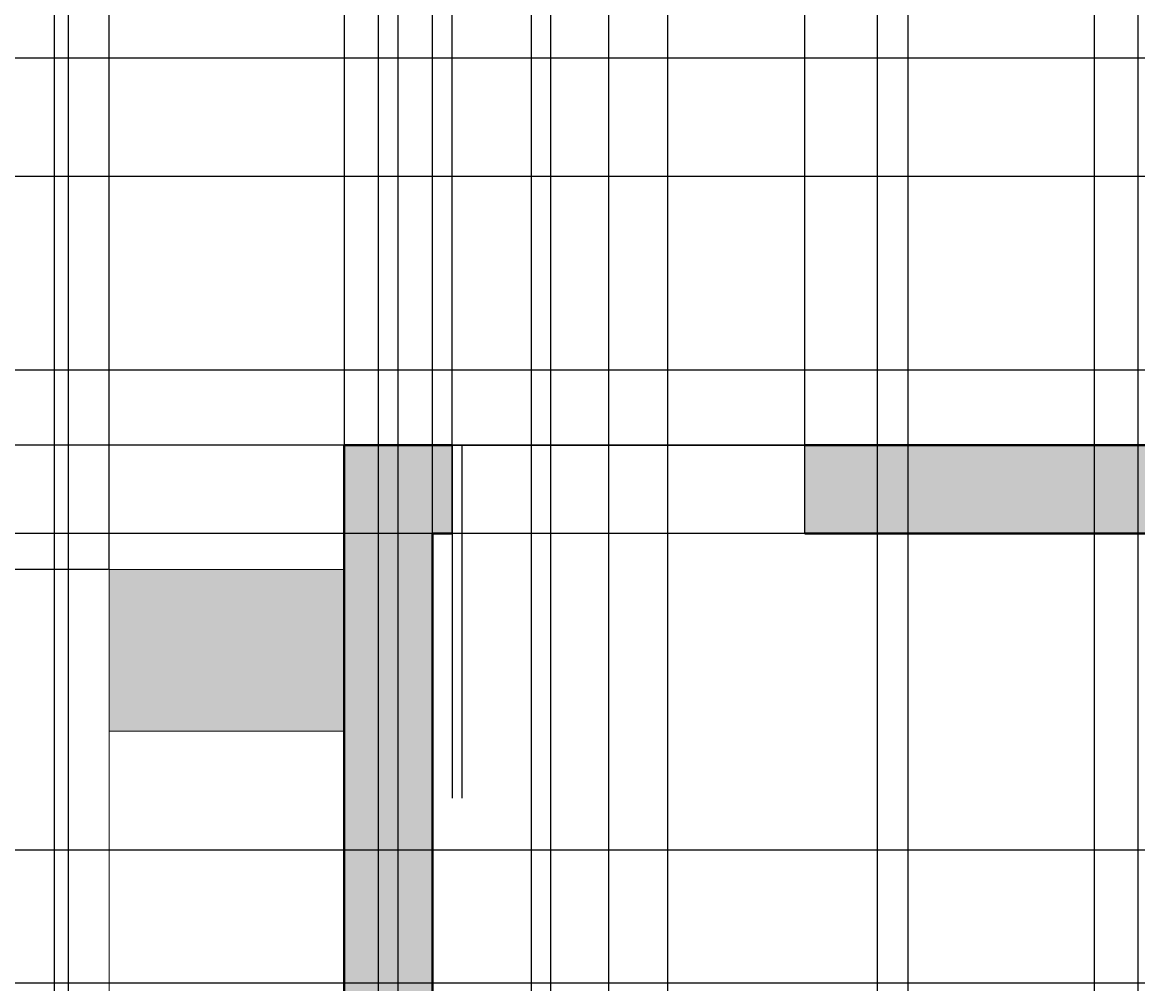
# Model space of a CAD drawing. Units: inches. Extents: x 818 to 1898, y 976 to 2364.
# Tile 27 of 96: x 1398 to 1512, y 1545 to 1643. Entities that reach past the tile are written whole.
import ezdxf

# ---------------------------------------------------------------- set-up
doc = ezdxf.new("R2010")
doc.units = ezdxf.units.IN
doc.header["$LTSCALE"] = 5
doc.header["$MEASUREMENT"] = 0
for name, color, linetype, lineweight in [('A-ANNO-DIMS', 2, 'Continuous', 18), ('A-DOOR', 3, 'Continuous', 25), ('A-FLOR-CASE', 8, 'Continuous', 18), ('A-FURN-PATT', 8, 'Continuous', 9), ('A-WALL', 7, 'Continuous', 40)]:
    doc.layers.add(name, color=color, linetype=linetype, lineweight=lineweight)
doc.layers.add('A-WALL-PATT', color=251, linetype='Continuous', lineweight=13, true_color=0x636466)
doc.styles.get("Standard").update_dxf_attribs({"font": 'arial.ttf'})
doc.dimstyles.get("Standard").update_dxf_attribs({"dimtxt": 0.18, "dimasz": 0.18, "dimexe": 0.18, "dimexo": 0.0625, "dimgap": 0.09, "dimtad": 0, "dimtih": 1, "dimtoh": 1, "dimdec": 4, "dimzin": 0, "dimdsep": 46, "dimtxsty": 'Standard', "dimcen": 0.09, "dimadec": 0, "dimazin": 0, "dimtfac": 1, "dimtdec": 4, "dimtofl": 0, "dimtmove": 0, "dimatfit": 3, "dimfxl": 1, "dimtolj": 1, "dimtzin": 0, "dimarcsym": 0})

# ---------------------------------------------------------------- blocks, each defined once
blk = doc.blocks.new('*D61')
at = {"layer": 'A-ANNO-DIMS', "color": 0, "lineweight": -2, "ltscale": 5, "transparency": 16777216}
for p, q in [((1071.73, 1203.03), (1071.73, 2363.87)), ((1071.91, 2363.69), (1250.94, 2363.69)), ((1430.55, 2363.69), (1251.51, 2363.69)), ((1430.73, 1203.03), (1430.73, 2363.87))]:
    blk.add_line(p, q, dxfattribs=at)
at = {"layer": 'A-ANNO-DIMS', "color": 0, "ltscale": 5, "transparency": 16777216}
for points in [[(1071.91, 2363.72), (1071.91, 2363.66), (1071.73, 2363.69)], [(1430.55, 2363.72), (1430.55, 2363.66), (1430.73, 2363.69)]]:
    blk.add_solid(points, dxfattribs=at)
at = {"layer": 'Defpoints', "color": 0, "ltscale": 5, "transparency": 16777216}
for p in [(1430.73, 2363.69), (1071.73, 1202.96), (1430.73, 1202.96)]:
    blk.add_point(p, dxfattribs=at)
at = {"layer": 'A-ANNO-DIMS', "color": 0, "ltscale": 5, "transparency": 16777216, "insert": (1251.23, 2363.69), "char_height": 0.18, "attachment_point": 5}
blk.add_mtext('\\A1;359', dxfattribs=at)
blk = doc.blocks.new('*D64')
at = {"layer": 'A-ANNO-DIMS', "color": 0, "lineweight": -2, "ltscale": 5, "transparency": 16777216}
for p, q in [((1197.73, 1501.14), (1197.73, 2363.87)), ((1197.91, 2363.69), (1313.93, 2363.69)), ((1430.55, 2363.69), (1314.52, 2363.69)), ((1430.73, 1501.14), (1430.73, 2363.87))]:
    blk.add_line(p, q, dxfattribs=at)
at = {"layer": 'A-ANNO-DIMS', "color": 0, "ltscale": 5, "transparency": 16777216}
for points in [[(1197.91, 2363.72), (1197.91, 2363.66), (1197.73, 2363.69)], [(1430.55, 2363.72), (1430.55, 2363.66), (1430.73, 2363.69)]]:
    blk.add_solid(points, dxfattribs=at)
at = {"layer": 'Defpoints', "color": 0, "ltscale": 5, "transparency": 16777216}
for p in [(1430.73, 2363.69), (1197.73, 1501.08), (1430.73, 1501.08)]:
    blk.add_point(p, dxfattribs=at)
at = {"layer": 'A-ANNO-DIMS', "color": 0, "ltscale": 5, "transparency": 16777216, "insert": (1314.23, 2363.69), "char_height": 0.18, "attachment_point": 5}
blk.add_mtext('\\A1;233', dxfattribs=at)
blk = doc.blocks.new('*D99')
at = {"layer": 'A-ANNO-DIMS', "color": 0, "lineweight": -2, "ltscale": 5, "transparency": 16777216}
for p, q in [((1391.88, 1071.12), (1391.88, 2363.87)), ((1392.06, 2363.69), (1420.45, 2363.69)), ((1449.64, 2363.69), (1421.24, 2363.69)), ((1449.82, 1071.12), (1449.82, 2363.87))]:
    blk.add_line(p, q, dxfattribs=at)
at = {"layer": 'A-ANNO-DIMS', "color": 0, "ltscale": 5, "transparency": 16777216}
for points in [[(1392.06, 2363.72), (1392.06, 2363.66), (1391.88, 2363.69)], [(1449.64, 2363.72), (1449.64, 2363.66), (1449.82, 2363.69)]]:
    blk.add_solid(points, dxfattribs=at)
at = {"layer": 'Defpoints', "color": 0, "ltscale": 5, "transparency": 16777216}
for p in [(1449.82, 2363.69), (1391.88, 1071.06), (1449.82, 1071.06)]:
    blk.add_point(p, dxfattribs=at)
at = {"layer": 'A-ANNO-DIMS', "color": 0, "ltscale": 5, "transparency": 16777216, "insert": (1420.85, 2363.69), "char_height": 0.18, "attachment_point": 5}
blk.add_mtext('\\A1;57.94', dxfattribs=at)
blk = doc.blocks.new('*D100')
at = {"layer": 'A-ANNO-DIMS', "color": 0, "lineweight": -2, "ltscale": 5, "transparency": 16777216}
for p, q in [((1449.82, 1071.12), (1449.82, 2363.87)), ((1450, 2363.69), (1478.17, 2363.69)), ((1507.12, 2363.69), (1478.95, 2363.69)), ((1507.3, 1071.12), (1507.3, 2363.87))]:
    blk.add_line(p, q, dxfattribs=at)
at = {"layer": 'A-ANNO-DIMS', "color": 0, "ltscale": 5, "transparency": 16777216}
for points in [[(1450, 2363.72), (1450, 2363.66), (1449.82, 2363.69)], [(1507.12, 2363.72), (1507.12, 2363.66), (1507.3, 2363.69)]]:
    blk.add_solid(points, dxfattribs=at)
at = {"layer": 'Defpoints', "color": 0, "ltscale": 5, "transparency": 16777216}
for p in [(1507.3, 2363.69), (1449.82, 1071.06), (1507.3, 1071.06)]:
    blk.add_point(p, dxfattribs=at)
at = {"layer": 'A-ANNO-DIMS', "color": 0, "ltscale": 5, "transparency": 16777216, "insert": (1478.56, 2363.69), "char_height": 0.18, "attachment_point": 5}
blk.add_mtext('\\A1;57.48', dxfattribs=at)
blk = doc.blocks.new('*D101')
at = {"layer": 'A-ANNO-DIMS', "color": 0, "lineweight": -2, "ltscale": 5, "transparency": 16777216}
for p, q in [((1507.3, 1071.12), (1507.3, 2363.87)), ((1507.48, 2363.69), (1536, 2363.69)), ((1565.3, 2363.69), (1536.78, 2363.69)), ((1565.48, 1071.12), (1565.48, 2363.87))]:
    blk.add_line(p, q, dxfattribs=at)
at = {"layer": 'A-ANNO-DIMS', "color": 0, "ltscale": 5, "transparency": 16777216}
for points in [[(1507.48, 2363.72), (1507.48, 2363.66), (1507.3, 2363.69)], [(1565.3, 2363.72), (1565.3, 2363.66), (1565.48, 2363.69)]]:
    blk.add_solid(points, dxfattribs=at)
at = {"layer": 'Defpoints', "color": 0, "ltscale": 5, "transparency": 16777216}
for p in [(1565.48, 2363.69), (1507.3, 1071.06), (1565.48, 1071.06)]:
    blk.add_point(p, dxfattribs=at)
at = {"layer": 'A-ANNO-DIMS', "color": 0, "ltscale": 5, "transparency": 16777216, "insert": (1536.39, 2363.69), "char_height": 0.18, "attachment_point": 5}
blk.add_mtext('\\A1;58.19', dxfattribs=at)
blk = doc.blocks.new('*D117')
at = {"layer": 'A-ANNO-DIMS', "color": 0, "lineweight": -2, "ltscale": 5, "transparency": 16777216}
for p, q in [((1766.29, 1545.18), (818.03, 1545.18)), ((818.21, 1545), (818.21, 1501.18)), ((818.21, 1456.99), (818.21, 1500.81)), ((1766.29, 1456.81), (818.03, 1456.81))]:
    blk.add_line(p, q, dxfattribs=at)
at = {"layer": 'A-ANNO-DIMS', "color": 0, "ltscale": 5, "transparency": 16777216}
for points in [[(818.18, 1545), (818.24, 1545), (818.21, 1545.18)], [(818.18, 1456.99), (818.24, 1456.99), (818.21, 1456.81)]]:
    blk.add_solid(points, dxfattribs=at)
at = {"layer": 'Defpoints', "color": 0, "ltscale": 5, "transparency": 16777216}
for p in [(818.21, 1545.18), (1766.35, 1545.18), (1766.35, 1456.81)]:
    blk.add_point(p, dxfattribs=at)
at = {"layer": 'A-ANNO-DIMS', "color": 0, "ltscale": 5, "transparency": 16777216, "insert": (818.21, 1501), "char_height": 0.18, "attachment_point": 5}
blk.add_mtext('\\A1;88.37', dxfattribs=at)
blk = doc.blocks.new('*D118')
at = {"layer": 'A-ANNO-DIMS', "color": 0, "lineweight": -2, "ltscale": 5, "transparency": 16777216}
for p, q in [((1766.29, 1627.51), (818.03, 1627.51)), ((818.21, 1627.33), (818.21, 1586.53)), ((818.21, 1545.36), (818.21, 1586.16)), ((1766.29, 1545.18), (818.03, 1545.18))]:
    blk.add_line(p, q, dxfattribs=at)
at = {"layer": 'A-ANNO-DIMS', "color": 0, "ltscale": 5, "transparency": 16777216}
for points in [[(818.18, 1627.33), (818.24, 1627.33), (818.21, 1627.51)], [(818.18, 1545.36), (818.24, 1545.36), (818.21, 1545.18)]]:
    blk.add_solid(points, dxfattribs=at)
at = {"layer": 'Defpoints', "color": 0, "ltscale": 5, "transparency": 16777216}
for p in [(818.21, 1627.51), (1766.35, 1627.51), (1766.35, 1545.18)]:
    blk.add_point(p, dxfattribs=at)
at = {"layer": 'A-ANNO-DIMS', "color": 0, "ltscale": 5, "transparency": 16777216, "insert": (818.21, 1586.34), "char_height": 0.18, "attachment_point": 5}
blk.add_mtext('\\A1;82.32', dxfattribs=at)
blk = doc.blocks.new('*D119')
at = {"layer": 'A-ANNO-DIMS', "color": 0, "lineweight": -2, "ltscale": 5, "transparency": 16777216}
for p, q in [((1766.29, 1716.99), (818.03, 1716.99)), ((818.21, 1716.81), (818.21, 1672.43)), ((818.21, 1627.69), (818.21, 1672.06)), ((1766.29, 1627.51), (818.03, 1627.51))]:
    blk.add_line(p, q, dxfattribs=at)
at = {"layer": 'A-ANNO-DIMS', "color": 0, "ltscale": 5, "transparency": 16777216}
for points in [[(818.18, 1716.81), (818.24, 1716.81), (818.21, 1716.99)], [(818.18, 1627.69), (818.24, 1627.69), (818.21, 1627.51)]]:
    blk.add_solid(points, dxfattribs=at)
at = {"layer": 'Defpoints', "color": 0, "ltscale": 5, "transparency": 16777216}
for p in [(818.21, 1716.99), (1766.35, 1716.99), (1766.35, 1627.51)]:
    blk.add_point(p, dxfattribs=at)
at = {"layer": 'A-ANNO-DIMS', "color": 0, "ltscale": 5, "transparency": 16777216, "insert": (818.21, 1672.25), "char_height": 0.18, "attachment_point": 5}
blk.add_mtext('\\A1;89.48', dxfattribs=at)
blk = doc.blocks.new('*D159')
at = {"layer": 'A-ANNO-DIMS', "color": 0, "lineweight": -2, "ltscale": 5, "transparency": 16777216}
for p, q in [((1206.73, 1687.02), (1206.73, 975.66)), ((1463.73, 1687.02), (1463.73, 975.66)), ((1206.91, 975.84), (1334.93, 975.84)), ((1463.55, 975.84), (1335.52, 975.84))]:
    blk.add_line(p, q, dxfattribs=at)
at = {"layer": 'A-ANNO-DIMS', "color": 0, "ltscale": 5, "transparency": 16777216}
for points in [[(1206.91, 975.87), (1206.91, 975.81), (1206.73, 975.84)], [(1463.55, 975.87), (1463.55, 975.81), (1463.73, 975.84)]]:
    blk.add_solid(points, dxfattribs=at)
at = {"layer": 'Defpoints', "color": 0, "ltscale": 5, "transparency": 16777216}
for p in [(1206.73, 1687.08), (1463.73, 1687.08), (1463.73, 975.84)]:
    blk.add_point(p, dxfattribs=at)
at = {"layer": 'A-ANNO-DIMS', "color": 0, "ltscale": 5, "transparency": 16777216, "insert": (1335.23, 975.84), "char_height": 0.18, "attachment_point": 5}
blk.add_mtext('\\A1;257', dxfattribs=at)
blk = doc.blocks.new('*D160')
at = {"layer": 'A-ANNO-DIMS', "color": 0, "lineweight": -2, "ltscale": 5, "transparency": 16777216}
for p, q in [((1463.73, 1687.02), (1463.73, 975.66)), ((1511.73, 1687.02), (1511.73, 975.66)), ((1463.91, 975.84), (1487.5, 975.84)), ((1511.55, 975.84), (1487.95, 975.84))]:
    blk.add_line(p, q, dxfattribs=at)
at = {"layer": 'A-ANNO-DIMS', "color": 0, "ltscale": 5, "transparency": 16777216}
for points in [[(1463.91, 975.87), (1463.91, 975.81), (1463.73, 975.84)], [(1511.55, 975.87), (1511.55, 975.81), (1511.73, 975.84)]]:
    blk.add_solid(points, dxfattribs=at)
at = {"layer": 'Defpoints', "color": 0, "ltscale": 5, "transparency": 16777216}
for p in [(1463.73, 1687.08), (1511.73, 1687.08), (1511.73, 975.84)]:
    blk.add_point(p, dxfattribs=at)
at = {"layer": 'A-ANNO-DIMS', "color": 0, "ltscale": 5, "transparency": 16777216, "insert": (1487.73, 975.84), "char_height": 0.18, "attachment_point": 5}
blk.add_mtext('\\A1;48', dxfattribs=at)
blk = doc.blocks.new('*D166')
at = {"layer": 'A-ANNO-DIMS', "color": 0, "lineweight": -2, "ltscale": 5, "transparency": 16777216}
for p, q in [((1401.15, 1510.14), (1401.15, 2363.87)), ((1401.33, 2363.69), (1415.54, 2363.69)), ((1430.55, 2363.69), (1416.33, 2363.69)), ((1430.73, 1510.14), (1430.73, 2363.87))]:
    blk.add_line(p, q, dxfattribs=at)
at = {"layer": 'A-ANNO-DIMS', "color": 0, "ltscale": 5, "transparency": 16777216}
for points in [[(1401.33, 2363.72), (1401.33, 2363.66), (1401.15, 2363.69)], [(1430.55, 2363.72), (1430.55, 2363.66), (1430.73, 2363.69)]]:
    blk.add_solid(points, dxfattribs=at)
at = {"layer": 'Defpoints', "color": 0, "ltscale": 5, "transparency": 16777216}
for p in [(1430.73, 2363.69), (1401.15, 1510.08), (1430.73, 1510.08)]:
    blk.add_point(p, dxfattribs=at)
at = {"layer": 'A-ANNO-DIMS', "color": 0, "ltscale": 5, "transparency": 16777216, "insert": (1415.94, 2363.69), "char_height": 0.18, "attachment_point": 5}
blk.add_mtext('\\A1;29.58', dxfattribs=at)
blk = doc.blocks.new('*D169')
at = {"layer": 'A-ANNO-DIMS', "color": 0, "lineweight": -2, "ltscale": 5, "transparency": 16777216}
for p, q in [((1441.73, 1600.14), (1441.73, 2363.87)), ((1441.91, 2363.69), (1459.51, 2363.69)), ((1477.55, 2363.69), (1459.94, 2363.69)), ((1477.73, 1600.14), (1477.73, 2363.87))]:
    blk.add_line(p, q, dxfattribs=at)
at = {"layer": 'A-ANNO-DIMS', "color": 0, "ltscale": 5, "transparency": 16777216}
for points in [[(1441.91, 2363.72), (1441.91, 2363.66), (1441.73, 2363.69)], [(1477.55, 2363.72), (1477.55, 2363.66), (1477.73, 2363.69)]]:
    blk.add_solid(points, dxfattribs=at)
at = {"layer": 'Defpoints', "color": 0, "ltscale": 5, "transparency": 16777216}
for p in [(1477.73, 2363.69), (1441.73, 1600.08), (1477.73, 1600.08)]:
    blk.add_point(p, dxfattribs=at)
at = {"layer": 'A-ANNO-DIMS', "color": 0, "ltscale": 5, "transparency": 16777216, "insert": (1459.73, 2363.69), "char_height": 0.18, "attachment_point": 5}
blk.add_mtext('\\A1;36', dxfattribs=at)
blk = doc.blocks.new('*D170')
at = {"layer": 'A-ANNO-DIMS', "color": 0, "lineweight": -2, "ltscale": 5, "transparency": 16777216}
for p, q in [((1430.79, 1600.08), (1897.92, 1600.08)), ((1897.74, 1599.9), (1897.74, 1550.76)), ((1897.74, 1501.26), (1897.74, 1550.4)), ((1430.79, 1501.08), (1897.92, 1501.08))]:
    blk.add_line(p, q, dxfattribs=at)
at = {"layer": 'A-ANNO-DIMS', "color": 0, "ltscale": 5, "transparency": 16777216}
for points in [[(1897.71, 1599.9), (1897.77, 1599.9), (1897.74, 1600.08)], [(1897.71, 1501.26), (1897.77, 1501.26), (1897.74, 1501.08)]]:
    blk.add_solid(points, dxfattribs=at)
at = {"layer": 'Defpoints', "color": 0, "ltscale": 5, "transparency": 16777216}
for p in [(1430.73, 1600.08), (1897.74, 1600.08), (1430.73, 1501.08)]:
    blk.add_point(p, dxfattribs=at)
at = {"layer": 'A-ANNO-DIMS', "color": 0, "ltscale": 5, "transparency": 16777216, "insert": (1897.74, 1550.58), "char_height": 0.18, "attachment_point": 5}
blk.add_mtext('\\A1;99', dxfattribs=at)
blk = doc.blocks.new('*D181')
at = {"layer": 'A-ANNO-DIMS', "color": 0, "lineweight": -2, "ltscale": 5, "transparency": 16777216}
for p, q in [((1599.66, 1639.58), (818.03, 1639.58)), ((818.21, 1639.4), (818.21, 1620.01)), ((818.21, 1600.26), (818.21, 1619.65)), ((1619.66, 1600.08), (818.03, 1600.08))]:
    blk.add_line(p, q, dxfattribs=at)
at = {"layer": 'A-ANNO-DIMS', "color": 0, "ltscale": 5, "transparency": 16777216}
for points in [[(818.18, 1639.4), (818.24, 1639.4), (818.21, 1639.58)], [(818.18, 1600.26), (818.24, 1600.26), (818.21, 1600.08)]]:
    blk.add_solid(points, dxfattribs=at)
at = {"layer": 'Defpoints', "color": 0, "ltscale": 5, "transparency": 16777216}
for p in [(1599.73, 1639.58), (818.21, 1600.08), (1619.73, 1600.08)]:
    blk.add_point(p, dxfattribs=at)
at = {"layer": 'A-ANNO-DIMS', "color": 0, "ltscale": 5, "transparency": 16777216, "insert": (818.21, 1619.83), "char_height": 0.18, "attachment_point": 5}
blk.add_mtext('\\A1;39.5', dxfattribs=at)
blk = doc.blocks.new('*D182')
at = {"layer": 'A-ANNO-DIMS', "color": 0, "lineweight": -2, "ltscale": 5, "transparency": 16777216}
for p, q in [((1463.73, 1687.02), (1463.73, 975.66)), ((1559.73, 1687.02), (1559.73, 975.66)), ((1463.91, 975.84), (1511.51, 975.84)), ((1559.55, 975.84), (1511.94, 975.84))]:
    blk.add_line(p, q, dxfattribs=at)
at = {"layer": 'A-ANNO-DIMS', "color": 0, "ltscale": 5, "transparency": 16777216}
for points in [[(1463.91, 975.87), (1463.91, 975.81), (1463.73, 975.84)], [(1559.55, 975.87), (1559.55, 975.81), (1559.73, 975.84)]]:
    blk.add_solid(points, dxfattribs=at)
at = {"layer": 'Defpoints', "color": 0, "ltscale": 5, "transparency": 16777216}
for p in [(1463.73, 1687.08), (1559.73, 1687.08), (1559.73, 975.84)]:
    blk.add_point(p, dxfattribs=at)
at = {"layer": 'A-ANNO-DIMS', "color": 0, "ltscale": 5, "transparency": 16777216, "insert": (1511.73, 975.84), "char_height": 0.18, "attachment_point": 5}
blk.add_mtext('\\A1;96', dxfattribs=at)
blk = doc.blocks.new('*D191')
at = {"layer": 'A-ANNO-DIMS', "color": 0, "lineweight": -2, "ltscale": 5, "transparency": 16777216}
for p, q in [((1434.23, 1409.11), (1434.23, 2363.87)), ((1434.41, 2363.69), (1435.08, 2363.69)), ((1436.05, 2363.69), (1435.37, 2363.69)), ((1436.23, 1409.11), (1436.23, 2363.87))]:
    blk.add_line(p, q, dxfattribs=at)
at = {"layer": 'A-ANNO-DIMS', "color": 0, "ltscale": 5, "transparency": 16777216}
for points in [[(1434.41, 2363.72), (1434.41, 2363.66), (1434.23, 2363.69)], [(1436.05, 2363.72), (1436.05, 2363.66), (1436.23, 2363.69)]]:
    blk.add_solid(points, dxfattribs=at)
at = {"layer": 'Defpoints', "color": 0, "ltscale": 5, "transparency": 16777216}
for p in [(1436.23, 2363.69), (1434.23, 1409.05), (1436.23, 1409.05)]:
    blk.add_point(p, dxfattribs=at)
at = {"layer": 'A-ANNO-DIMS', "color": 0, "ltscale": 5, "transparency": 16777216, "insert": (1435.23, 2363.69), "char_height": 0.18, "attachment_point": 5}
blk.add_mtext('\\A1;2', dxfattribs=at)
blk = doc.blocks.new('*D194')
at = {"layer": 'A-ANNO-DIMS', "color": 0, "lineweight": -2, "ltscale": 5, "transparency": 16777216}
for p, q in [((1616.66, 1591.08), (818.03, 1591.08)), ((818.21, 1590.9), (818.21, 1575.1)), ((818.21, 1558.93), (818.21, 1574.73)), ((1616.66, 1558.75), (818.03, 1558.75))]:
    blk.add_line(p, q, dxfattribs=at)
at = {"layer": 'A-ANNO-DIMS', "color": 0, "ltscale": 5, "transparency": 16777216}
for points in [[(818.18, 1590.9), (818.24, 1590.9), (818.21, 1591.08)], [(818.18, 1558.93), (818.24, 1558.93), (818.21, 1558.75)]]:
    blk.add_solid(points, dxfattribs=at)
at = {"layer": 'Defpoints', "color": 0, "ltscale": 5, "transparency": 16777216}
for p in [(818.21, 1591.08), (1616.73, 1591.08), (1616.73, 1558.75)]:
    blk.add_point(p, dxfattribs=at)
at = {"layer": 'A-ANNO-DIMS', "color": 0, "ltscale": 5, "transparency": 16777216, "insert": (818.21, 1574.92), "char_height": 0.18, "attachment_point": 5}
blk.add_mtext('\\A1;32.326', dxfattribs=at)
blk = doc.blocks.new('*D196')
at = {"layer": 'A-ANNO-DIMS', "color": 0, "lineweight": -2, "ltscale": 5, "transparency": 16777216}
for p, q in [((1439.73, 1526.73), (1439.73, 2363.87)), ((1439.91, 2363.69), (1448.51, 2363.69)), ((1457.55, 2363.69), (1448.94, 2363.69)), ((1457.73, 1526.73), (1457.73, 2363.87))]:
    blk.add_line(p, q, dxfattribs=at)
at = {"layer": 'A-ANNO-DIMS', "color": 0, "ltscale": 5, "transparency": 16777216}
for points in [[(1439.91, 2363.72), (1439.91, 2363.66), (1439.73, 2363.69)], [(1457.55, 2363.72), (1457.55, 2363.66), (1457.73, 2363.69)]]:
    blk.add_solid(points, dxfattribs=at)
at = {"layer": 'Defpoints', "color": 0, "ltscale": 5, "transparency": 16777216}
for p in [(1457.73, 2363.69), (1439.73, 1526.67), (1457.73, 1526.67)]:
    blk.add_point(p, dxfattribs=at)
at = {"layer": 'A-ANNO-DIMS', "color": 0, "ltscale": 5, "transparency": 16777216, "insert": (1448.73, 2363.69), "char_height": 0.18, "attachment_point": 5}
blk.add_mtext('\\A1;18', dxfattribs=at)
blk = doc.blocks.new('*D214')
at = {"layer": 'A-ANNO-DIMS', "color": 0, "lineweight": -2, "ltscale": 5, "transparency": 16777216}
for p, q in [((1511.73, 1687.02), (1511.73, 975.66)), ((1714.73, 1687.02), (1714.73, 975.66)), ((1511.91, 975.84), (1612.93, 975.84)), ((1714.55, 975.84), (1613.52, 975.84))]:
    blk.add_line(p, q, dxfattribs=at)
at = {"layer": 'A-ANNO-DIMS', "color": 0, "ltscale": 5, "transparency": 16777216}
for points in [[(1511.91, 975.87), (1511.91, 975.81), (1511.73, 975.84)], [(1714.55, 975.87), (1714.55, 975.81), (1714.73, 975.84)]]:
    blk.add_solid(points, dxfattribs=at)
at = {"layer": 'Defpoints', "color": 0, "ltscale": 5, "transparency": 16777216}
for p in [(1511.73, 1687.08), (1714.73, 1687.08), (1714.73, 975.84)]:
    blk.add_point(p, dxfattribs=at)
at = {"layer": 'A-ANNO-DIMS', "color": 0, "ltscale": 5, "transparency": 16777216, "insert": (1613.23, 975.84), "char_height": 0.18, "attachment_point": 5}
blk.add_mtext('\\A1;203', dxfattribs=at)
blk = doc.blocks.new('*D231')
at = {"layer": 'A-ANNO-DIMS', "color": 0, "lineweight": -2, "ltscale": 5, "transparency": 16777216}
for p, q in [((1303.93, 1952.98), (1303.93, 975.66)), ((1402.52, 1952.98), (1402.52, 975.66)), ((1304.11, 975.84), (1352.83, 975.84)), ((1402.34, 975.84), (1353.62, 975.84))]:
    blk.add_line(p, q, dxfattribs=at)
at = {"layer": 'A-ANNO-DIMS', "color": 0, "ltscale": 5, "transparency": 16777216}
for points in [[(1304.11, 975.87), (1304.11, 975.81), (1303.93, 975.84)], [(1402.34, 975.87), (1402.34, 975.81), (1402.52, 975.84)]]:
    blk.add_solid(points, dxfattribs=at)
at = {"layer": 'Defpoints', "color": 0, "ltscale": 5, "transparency": 16777216}
for p in [(1303.93, 1953.04), (1402.52, 1953.04), (1402.52, 975.84)]:
    blk.add_point(p, dxfattribs=at)
at = {"layer": 'A-ANNO-DIMS', "color": 0, "ltscale": 5, "transparency": 16777216, "insert": (1353.22, 975.84), "char_height": 0.18, "attachment_point": 5}
blk.add_mtext('\\A1;98.59', dxfattribs=at)
blk = doc.blocks.new('*D242')
at = {"layer": 'A-ANNO-DIMS', "color": 0, "lineweight": -2, "ltscale": 5, "transparency": 16777216}
for p, q in [((1488.26, 1948.6), (1488.26, 975.66)), ((1513.23, 1948.6), (1513.23, 975.66)), ((1488.44, 975.84), (1500.35, 975.84)), ((1513.05, 975.84), (1501.14, 975.84))]:
    blk.add_line(p, q, dxfattribs=at)
at = {"layer": 'A-ANNO-DIMS', "color": 0, "ltscale": 5, "transparency": 16777216}
for points in [[(1488.44, 975.87), (1488.44, 975.81), (1488.26, 975.84)], [(1513.05, 975.87), (1513.05, 975.81), (1513.23, 975.84)]]:
    blk.add_solid(points, dxfattribs=at)
at = {"layer": 'Defpoints', "color": 0, "ltscale": 5, "transparency": 16777216}
for p in [(1488.26, 1948.66), (1513.23, 1948.66), (1513.23, 975.84)]:
    blk.add_point(p, dxfattribs=at)
at = {"layer": 'A-ANNO-DIMS', "color": 0, "ltscale": 5, "transparency": 16777216, "insert": (1500.74, 975.84), "char_height": 0.18, "attachment_point": 5}
blk.add_mtext('\\A1;24.97', dxfattribs=at)
blk = doc.blocks.new('*D243')
at = {"layer": 'A-ANNO-DIMS', "color": 0, "lineweight": -2, "ltscale": 5, "transparency": 16777216}
for p, q in [((1451.77, 2020.02), (1451.77, 975.66)), ((1590.73, 2020.02), (1590.73, 975.66)), ((1451.95, 975.84), (1520.79, 975.84)), ((1590.55, 975.84), (1521.7, 975.84))]:
    blk.add_line(p, q, dxfattribs=at)
at = {"layer": 'A-ANNO-DIMS', "color": 0, "ltscale": 5, "transparency": 16777216}
for points in [[(1451.95, 975.87), (1451.95, 975.81), (1451.77, 975.84)], [(1590.55, 975.87), (1590.55, 975.81), (1590.73, 975.84)]]:
    blk.add_solid(points, dxfattribs=at)
at = {"layer": 'Defpoints', "color": 0, "ltscale": 5, "transparency": 16777216}
for p in [(1451.77, 2020.08), (1590.73, 2020.08), (1590.73, 975.84)]:
    blk.add_point(p, dxfattribs=at)
at = {"layer": 'A-ANNO-DIMS', "color": 0, "ltscale": 5, "transparency": 16777216, "insert": (1521.25, 975.84), "char_height": 0.18, "attachment_point": 5}
blk.add_mtext('\\A1;138.96', dxfattribs=at)
blk = doc.blocks.new('*D253')
at = {"layer": 'A-ANNO-DIMS', "color": 0, "lineweight": -2, "ltscale": 5, "transparency": 16777216}
for p, q in [((1485.12, 2053.02), (1485.12, 975.66)), ((1538.52, 2053.02), (1538.52, 975.66)), ((1485.3, 975.84), (1511.42, 975.84)), ((1538.34, 975.84), (1512.21, 975.84))]:
    blk.add_line(p, q, dxfattribs=at)
at = {"layer": 'A-ANNO-DIMS', "color": 0, "ltscale": 5, "transparency": 16777216}
for points in [[(1485.3, 975.87), (1485.3, 975.81), (1485.12, 975.84)], [(1538.34, 975.87), (1538.34, 975.81), (1538.52, 975.84)]]:
    blk.add_solid(points, dxfattribs=at)
at = {"layer": 'Defpoints', "color": 0, "ltscale": 5, "transparency": 16777216}
for p in [(1485.12, 2053.08), (1538.52, 2053.08), (1538.52, 975.84)]:
    blk.add_point(p, dxfattribs=at)
at = {"layer": 'A-ANNO-DIMS', "color": 0, "ltscale": 5, "transparency": 16777216, "insert": (1511.82, 975.84), "char_height": 0.18, "attachment_point": 5}
blk.add_mtext('\\A1;53.39', dxfattribs=at)
blk = doc.blocks.new('*D272')
at = {"layer": 'A-ANNO-DIMS', "color": 0, "lineweight": -2, "ltscale": 5, "transparency": 16777216}
for p, q in [((1406.66, 1587.42), (818.03, 1587.42)), ((818.21, 1587.24), (818.21, 1556.89)), ((818.21, 1526.18), (818.21, 1556.52)), ((1406.66, 1526), (818.03, 1526))]:
    blk.add_line(p, q, dxfattribs=at)
at = {"layer": 'A-ANNO-DIMS', "color": 0, "ltscale": 5, "transparency": 16777216}
for points in [[(818.18, 1587.24), (818.24, 1587.24), (818.21, 1587.42)], [(818.18, 1526.18), (818.24, 1526.18), (818.21, 1526)]]:
    blk.add_solid(points, dxfattribs=at)
at = {"layer": 'Defpoints', "color": 0, "ltscale": 5, "transparency": 16777216}
for p in [(818.21, 1587.42), (1406.73, 1587.42), (1406.73, 1526)]:
    blk.add_point(p, dxfattribs=at)
at = {"layer": 'A-ANNO-DIMS', "color": 0, "ltscale": 5, "transparency": 16777216, "insert": (818.21, 1556.71), "char_height": 0.18, "attachment_point": 5}
blk.add_mtext('\\A1;61.42', dxfattribs=at)
blk = doc.blocks.new('*D273')
at = {"layer": 'A-ANNO-DIMS', "color": 0, "lineweight": -2, "ltscale": 5, "transparency": 16777216}
for p, q in [((1406.73, 1587.48), (1406.73, 2363.87)), ((1406.91, 2363.69), (1418.51, 2363.69)), ((1430.55, 2363.69), (1418.95, 2363.69)), ((1430.73, 1587.48), (1430.73, 2363.87))]:
    blk.add_line(p, q, dxfattribs=at)
at = {"layer": 'A-ANNO-DIMS', "color": 0, "ltscale": 5, "transparency": 16777216}
for points in [[(1406.91, 2363.72), (1406.91, 2363.66), (1406.73, 2363.69)], [(1430.55, 2363.72), (1430.55, 2363.66), (1430.73, 2363.69)]]:
    blk.add_solid(points, dxfattribs=at)
at = {"layer": 'Defpoints', "color": 0, "ltscale": 5, "transparency": 16777216}
for p in [(1430.73, 2363.69), (1406.73, 1587.42), (1430.73, 1587.42)]:
    blk.add_point(p, dxfattribs=at)
at = {"layer": 'A-ANNO-DIMS', "color": 0, "ltscale": 5, "transparency": 16777216, "insert": (1418.73, 2363.69), "char_height": 0.18, "attachment_point": 5}
blk.add_mtext('\\A1;24', dxfattribs=at)
blk = doc.blocks.new('*D291')
at = {"layer": 'A-ANNO-DIMS', "color": 0, "lineweight": -2, "ltscale": 5, "transparency": 16777216}
for p, q in [((1206.79, 1687.08), (1897.92, 1687.08)), ((1897.74, 1686.9), (1897.74, 1647.61)), ((1897.74, 1607.95), (1897.74, 1647.24)), ((1318.96, 1607.77), (1897.92, 1607.77))]:
    blk.add_line(p, q, dxfattribs=at)
at = {"layer": 'A-ANNO-DIMS', "color": 0, "ltscale": 5, "transparency": 16777216}
for points in [[(1897.71, 1686.9), (1897.77, 1686.9), (1897.74, 1687.08)], [(1897.71, 1607.95), (1897.77, 1607.95), (1897.74, 1607.77)]]:
    blk.add_solid(points, dxfattribs=at)
at = {"layer": 'Defpoints', "color": 0, "ltscale": 5, "transparency": 16777216}
for p in [(1206.73, 1687.08), (1897.74, 1687.08), (1318.89, 1607.77)]:
    blk.add_point(p, dxfattribs=at)
at = {"layer": 'A-ANNO-DIMS', "color": 0, "ltscale": 5, "transparency": 16777216, "insert": (1897.74, 1647.42), "char_height": 0.18, "attachment_point": 5}
blk.add_mtext('\\A1;79.3', dxfattribs=at)

msp = doc.modelspace()

# ---------------------------------------------------------------- hatches: boundary and pattern name
at = {"layer": 'A-FURN-PATT', "ltscale": 5}
h = msp.add_hatch(color=256, dxfattribs=at)
h.dxf.hatch_style = 1
h.paths.add_polyline_path([(1336.7936, 1953.0408), (1314.2595, 1953.0408), (1314.2595, 1941.0096), (1336.7936, 1941.0096)])
h.paths.add_polyline_path([(1338.9915, 1941.0096), (1336.7936, 1941.0096), (1336.7936, 1937.7177), (1314.2595, 1937.7177), (1314.2595, 1941.0096), (1310.9077, 1941.0096), (1310.9077, 1935.2252), (1338.9915, 1935.2252)])
h.paths.add_polyline_path([(1336.7936, 1941.0096), (1314.2595, 1941.0096), (1314.2595, 1937.7177), (1336.7936, 1937.7177)], flags=17)
h.paths.add_polyline_path([(1367.9307, 1959.6079), (1345.3966, 1959.6079), (1345.3966, 1941.0096), (1367.9307, 1941.0096)])
h.paths.add_polyline_path([(1398.8475, 1953.0408), (1376.3134, 1953.0408), (1376.3134, 1952.6393), (1390.1242, 1941.0096), (1398.8475, 1941.0096)])
h.paths.add_polyline_path([(1376.3134, 1952.6393), (1376.3134, 1941.0096), (1390.1242, 1941.0096)], flags=17)
h.paths.add_polyline_path([(1370.1286, 1941.0096), (1367.9307, 1941.0096), (1367.9307, 1937.7177), (1345.3966, 1937.7177), (1345.3966, 1941.0096), (1342.0448, 1941.0096), (1342.0448, 1935.2252), (1370.1286, 1935.2252)])
h.paths.add_polyline_path([(1367.9307, 1941.0096), (1345.3966, 1941.0096), (1345.3966, 1937.7177), (1367.9307, 1937.7177)], flags=17)
h.paths.add_polyline_path([(1390.1242, 1941.0096), (1376.3134, 1941.0096), (1376.3134, 1937.7177), (1394.0336, 1937.7177)], flags=17)
h.paths.add_polyline_path([(1394.0336, 1937.7177), (1376.3134, 1937.7177), (1376.3134, 1941.0096), (1372.9616, 1941.0096), (1372.9616, 1935.2252), (1396.9935, 1935.2252)])
h.paths.add_polyline_path([(1398.8475, 1941.0096), (1390.1242, 1941.0096), (1394.0336, 1937.7177), (1398.8475, 1937.7177)])
h.paths.add_polyline_path([(1401.0455, 1941.0096), (1398.8475, 1941.0096), (1398.8475, 1937.7177), (1394.0336, 1937.7177), (1396.9935, 1935.2252), (1401.0455, 1935.2252)])
h.paths.add_polyline_path([(1336.7936, 2020.4229), (1314.2595, 2020.4229), (1314.2595, 2008.3917), (1336.7936, 2008.3917)])
h.paths.add_polyline_path([(1336.7936, 2023.7149), (1314.2595, 2023.7149), (1314.2595, 2020.4229), (1336.7936, 2020.4229)], flags=17)
h.paths.add_polyline_path([(1338.9915, 2026.2074), (1310.9077, 2026.2074), (1310.9077, 2020.4229), (1314.2595, 2020.4229), (1314.2595, 2023.7149), (1336.7936, 2023.7149), (1336.7936, 2020.4229), (1338.9915, 2020.4229)])
h.paths.add_polyline_path([(1367.9307, 2023.7149), (1345.3966, 2023.7149), (1345.3966, 2020.4229), (1367.9307, 2020.4229)], flags=17)
h.paths.add_polyline_path([(1370.1286, 2026.2074), (1342.0448, 2026.2074), (1342.0448, 2020.4229), (1345.3966, 2020.4229), (1345.3966, 2023.7149), (1367.9307, 2023.7149), (1367.9307, 2020.4229), (1370.1286, 2020.4229)])
h.paths.add_polyline_path([(1367.9307, 2020.4229), (1345.3966, 2020.4229), (1345.3966, 2008.3917), (1367.9307, 2008.3917)])
h.paths.add_polyline_path([(1398.8475, 2020.4229), (1388.1824, 2020.4229), (1376.3134, 2010.4284), (1376.3134, 2008.3917), (1398.8475, 2008.3917)])
h.paths.add_polyline_path([(1392.0918, 2023.7149), (1376.3134, 2023.7149), (1376.3134, 2020.4229), (1388.1824, 2020.4229)], flags=17)
h.paths.add_polyline_path([(1388.1824, 2020.4229), (1376.3134, 2020.4229), (1376.3134, 2010.4284)], flags=17)
h.paths.add_polyline_path([(1395.0518, 2026.2074), (1372.9616, 2026.2074), (1372.9616, 2020.4229), (1376.3134, 2020.4229), (1376.3134, 2023.7149), (1392.0918, 2023.7149)])
h.paths.add_polyline_path([(1398.8475, 2023.7149), (1392.0918, 2023.7149), (1388.1824, 2020.4229), (1398.8475, 2020.4229)])
h.paths.add_polyline_path([(1401.0455, 2026.2074), (1395.0518, 2026.2074), (1392.0918, 2023.7149), (1398.8475, 2023.7149), (1398.8475, 2020.4229), (1401.0455, 2020.4229)])
h.paths.add_polyline_path([(1327.0339, 1897.8663), (1311.025, 1897.8663), (1311.025, 1876.0782), (1327.0339, 1876.0782)])
h.paths.add_polyline_path([(1377.7791, 1897.8663), (1359.9579, 1897.8663), (1359.9579, 1876.0782), (1377.7791, 1876.0782)])
h.paths.add_polyline_path([(1430.7251, 1541.0439), (1406.7251, 1541.0439), (1406.7251, 1525.9965), (1430.7251, 1525.9965)])
h.paths.add_polyline_path([(1430.7251, 1587.4164), (1406.7251, 1587.4164), (1406.7251, 1570.9187), (1430.7251, 1570.9187)])
at = {"layer": 'A-WALL-PATT', "ltscale": 5}
h = msp.add_hatch(color=256, dxfattribs=at)
h.dxf.hatch_style = 1
h.paths.add_polyline_path([(1267.7252, 1928.9218), (1258.7252, 1928.9218), (1258.7252, 1913.6401), (1250.3029, 1913.6401), (1250.3029, 1878.3919), (1258.7252, 1878.3919), (1258.7252, 1862.9652), (1267.7252, 1862.9652)])
h.paths.add_polyline_path([(1267.7252, 1814.9652), (1258.7252, 1814.9652), (1258.7252, 1755.3321), (1267.7252, 1755.3321)])
h.paths.add_polyline_path([(1463.7251, 1696.0782), (1267.7252, 1696.0782), (1267.7252, 1707.3321), (1258.7252, 1707.3321), (1258.7252, 1700.0782), (1251.9333, 1700.0782), (1251.9333, 1687.0782), (1463.7251, 1687.0782)])
h.paths.add_polyline_path([(1714.7251, 1717.3178), (1705.7252, 1717.3178), (1705.7252, 1696.0782), (1599.7251, 1696.0782), (1599.7251, 1790.0782), (1705.7252, 1790.0782), (1705.7252, 1785.6125), (1714.7251, 1785.6125), (1714.7251, 1827.2125), (1705.7252, 1827.2125), (1705.7252, 1802.0782), (1599.7251, 1802.0782), (1599.7251, 1867.0782), (1705.7252, 1867.0782), (1705.7252, 1857.2125), (1714.7251, 1857.2125), (1714.7251, 1930.0316), (1741.8409, 1930.0316), (1741.8409, 1935.0316), (1714.7251, 1935.0316), (1714.7251, 1957.0338), (1741.8409, 1957.0338), (1741.8409, 1962.0338), (1714.7251, 1962.0338), (1705.7252, 1962.0338), (1705.7252, 1948.0782), (1599.7251, 1948.0782), (1599.7251, 1981.0782), (1590.7251, 1981.0782), (1590.7251, 1941.0782), (1620.7252, 1941.0782), (1705.7252, 1941.0782), (1705.7252, 1876.0782), (1599.7251, 1876.0782), (1599.7251, 1911.0782), (1590.7251, 1911.0782), (1590.7251, 1876.0782), (1429.2252, 1876.0782), (1429.2252, 1867.0782), (1511.7251, 1867.0782), (1528.593, 1867.0782), (1595.7252, 1867.0782), (1595.7252, 1773.0782), (1520.7252, 1773.0782), (1520.7252, 1837.5823), (1532.593, 1837.5823), (1532.593, 1867.0782), (1528.593, 1867.0782), (1528.593, 1841.5823), (1511.7251, 1841.5823), (1511.7251, 1744.9714), (1520.7252, 1744.9714), (1520.7252, 1761.0782), (1595.7252, 1761.0782), (1595.7252, 1696.0782), (1520.7252, 1696.0782), (1520.7252, 1716.0454), (1511.7251, 1716.0454), (1511.7251, 1696.0782), (1511.7251, 1687.0782), (1714.7251, 1687.0782)])
h.paths.add_polyline_path([(1714.7251, 2053.0782), (1714.7251, 2081.1881), (1709.7252, 2081.1881), (1709.7252, 2053.0782), (1681.6446, 2053.0782), (1681.6446, 2081.1881), (1676.6446, 2081.1881), (1676.6446, 2053.0782), (1538.5155, 2053.0782), (1538.5155, 2044.0782), (1590.7251, 2044.0782), (1590.7251, 2011.0782), (1599.7251, 2011.0782), (1599.7251, 2044.0782), (1705.7252, 2044.0782), (1705.7252, 2014.5114), (1714.7251, 2014.5114)])
h.paths.add_polyline_path([(1485.1216, 2053.0782), (1422.02, 2053.0782), (1422.02, 2081.1881), (1413.02, 2081.1881), (1413.02, 2053.0782), (1399.6356, 2053.0782), (1399.6356, 2081.1881), (1390.6356, 2081.1881), (1390.6356, 2053.0782), (1388.0315, 2053.0782), (1388.0315, 2044.0782), (1416.2743, 2044.0782), (1485.1216, 2044.0782)])
h.paths.add_polyline_path([(1330.305, 2053.0782), (1258.7252, 2053.0782), (1258.7252, 2019.2871), (1267.7252, 2019.2871), (1267.7252, 2044.0782), (1330.305, 2044.0782)])
h.paths.add_polyline_path([(1258.7252, 2053.0782), (1214.6577, 2053.0782), (1214.6577, 2044.0782), (1258.7252, 2044.0782)])
h.paths.add_polyline_path([(1214.6577, 2053.0782), (1180.349, 2053.0782), (1180.349, 2044.0782), (1214.6577, 2044.0782)])
h.paths.add_polyline_path([(1714.7251, 1639.5782), (1741.8409, 1639.5782), (1741.8409, 1643.5782), (1714.7251, 1643.5782), (1714.7251, 1649.9029), (1705.7252, 1649.9029), (1705.7252, 1600.0782), (1477.7251, 1600.0782), (1477.7251, 1591.0782), (1520.7252, 1591.0782), (1616.7251, 1591.0782), (1616.7251, 1416.6857), (1622.7252, 1416.6857), (1622.7252, 1463.0782), (1624.7252, 1463.0782), (1624.7252, 1467.0782), (1622.7252, 1467.0782), (1622.7252, 1591.0782), (1705.7252, 1591.0782), (1705.7252, 1545.0782), (1714.7251, 1545.0782), (1741.8409, 1545.0782), (1741.8409, 1549.0782), (1714.7251, 1549.0782), (1714.7251, 1593.9175), (1737.8409, 1593.9175), (1737.8409, 1597.9175), (1714.7251, 1597.9175)])
h.paths.add_polyline_path([(1674.9024, 2060.7419), (1714.7045, 2060.7419), (1714.7045, 2073.1061), (1674.9024, 2073.1061)], flags=25)
h.paths.add_polyline_path([(1394.5468, 2061.6618), (1422.2344, 2061.6618), (1422.2344, 2074.0261), (1394.5468, 2074.0261)], flags=24)
h = msp.add_hatch(color=256, dxfattribs=at)
h.dxf.hatch_style = 1
h.paths.add_polyline_path([(1206.7251, 1687.0782), (1206.7251, 1700.0782), (1197.7251, 1700.0782), (1197.7251, 1501.0782), (1206.7251, 1501.0782), (1206.7251, 1510.0782)])
h.paths.add_polyline_path([(1197.7251, 1590.7585), (1173.7252, 1590.7585), (1173.7252, 1586.7585), (1197.7251, 1586.7585)])
h.paths.add_polyline_path([(1197.7251, 1534.6024), (1173.7252, 1534.6024), (1173.7252, 1530.6024), (1197.7251, 1530.6024)])
h.paths.add_polyline_path([(1365.1463, 1510.0782), (1283.8183, 1510.0782), (1283.8183, 1501.0782), (1365.1463, 1501.0782)])
h.paths.add_polyline_path([(1439.7251, 1591.0782), (1441.7251, 1591.0782), (1441.7251, 1600.0782), (1430.7251, 1600.0782), (1430.7251, 1510.0782), (1406.7251, 1510.0782), (1401.1463, 1510.0782), (1401.1463, 1501.0782), (1430.7251, 1501.0782), (1430.7251, 1486.2383), (1430.7251, 1409.0522), (1439.7251, 1409.0522)])

# ---------------------------------------------------------------- linework, layer by layer
at = {"layer": 'A-DOOR'}
for p, q in [((1441.7251, 1591.0782), (1441.7251, 1600.0782)), ((1441.7251, 1600.0782), (1441.7251, 1564.0782)), ((1442.7252, 1600.0782), (1442.7252, 1564.0782)), ((1477.7251, 1591.0782), (1477.7251, 1600.0782))]:
    msp.add_line(p, q, dxfattribs=at)
at = {"layer": 'A-FLOR-CASE'}
for p, q in [((1406.7251, 1525.9965), (1406.7251, 1587.4164)), ((1406.7251, 1587.4164), (1430.7251, 1587.4164))]:
    msp.add_line(p, q, dxfattribs=at)
msp.add_lwpolyline([(1406.7251, 1570.9187), (1430.7251, 1570.9187), (1430.7251, 1541.0439), (1406.7251, 1541.0439)], close=True, dxfattribs=at)
at = {"layer": 'A-WALL'}
for p, q in [((1430.7251, 1600.0782), (1430.7251, 1510.0782)), ((1430.7251, 1600.0782), (1441.7251, 1600.0782)), ((1477.7251, 1600.0782), (1705.7252, 1600.0782)), ((1439.7251, 1591.0782), (1439.7251, 1355.0782)), ((1439.7251, 1591.0782), (1441.7251, 1591.0782)), ((1477.7251, 1591.0782), (1520.7252, 1591.0782))]:
    msp.add_line(p, q, dxfattribs=at)

# ---------------------------------------------------------------- dimensions: what is measured, and where the dimension line sits
at = {"layer": 'A-ANNO-DIMS', "ltscale": 5}
for base, p1, p2, override, picture, middle in [((1430.7251, 2363.6929), (1071.7251, 1202.9642), (1430.7251, 1202.9642), {"dimdec": 0, "dimlfac": 1, "dimrnd": 0, "dimzin": 0, "dimdsep": 46, "dimlunit": 2}, '*D61', (1251.2251, 2363.6929)), ((1430.7251, 2363.6929), (1197.7251, 1501.0782), (1430.7251, 1501.0782), {"dimdec": 0, "dimlfac": 1, "dimrnd": 0, "dimzin": 0, "dimdsep": 46, "dimlunit": 2}, '*D64', (1314.2251, 2363.6929)), ((1449.8196, 2363.6929), (1391.8757, 1071.0552), (1449.8196, 1071.0552), {"dimdec": 2, "dimlfac": 1, "dimrnd": 0, "dimzin": 0, "dimdsep": 46, "dimlunit": 2}, '*D99', (1420.8477, 2363.6929)), ((1430.7251, 2363.6929), (1401.1463, 1510.0782), (1430.7251, 1510.0782), {"dimdec": 2, "dimlfac": 1, "dimrnd": 0, "dimzin": 0, "dimdsep": 46, "dimlunit": 2}, '*D166', (1415.9357, 2363.6929)), ((1430.7251, 2363.6929), (1406.7251, 1587.4164), (1430.7251, 1587.4164), {"dimdec": 0, "dimlfac": 1, "dimrnd": 0, "dimzin": 0, "dimdsep": 46, "dimlunit": 2}, '*D273', (1418.7251, 2363.6929)), ((1436.2251, 2363.6929), (1434.2251, 1409.0522), (1436.2251, 1409.0522), {"dimdec": 0, "dimlfac": 1, "dimrnd": 0, "dimzin": 0, "dimdsep": 46, "dimlunit": 2}, '*D191', (1435.2251, 2363.6929)), ((1457.7251, 2363.6929), (1439.7251, 1526.6712), (1457.7251, 1526.6712), {"dimdec": 0, "dimlfac": 1, "dimrnd": 0, "dimzin": 0, "dimdsep": 46, "dimlunit": 2}, '*D196', (1448.7251, 2363.6929)), ((1477.7251, 2363.6929), (1441.7251, 1600.0782), (1477.7251, 1600.0782), {"dimdec": 0, "dimlfac": 1, "dimrnd": 0, "dimzin": 0, "dimdsep": 46, "dimlunit": 2}, '*D169', (1459.7251, 2363.6929)), ((1507.2982, 2363.6929), (1449.8196, 1071.0552), (1507.2982, 1071.0552), {"dimdec": 2, "dimlfac": 1, "dimrnd": 0, "dimzin": 0, "dimdsep": 46, "dimlunit": 2}, '*D100', (1478.5589, 2363.6929)), ((1565.4835, 2363.6929), (1507.2982, 1071.0552), (1565.4835, 1071.0552), {"dimdec": 2, "dimlfac": 1, "dimrnd": 0, "dimzin": 0, "dimdsep": 46, "dimlunit": 2}, '*D101', (1536.3908, 2363.6929)), ((1538.5155, 975.8433), (1485.1216, 2053.0782), (1538.5155, 2053.0782), {"dimdec": 2, "dimlfac": 1, "dimrnd": 0, "dimzin": 0, "dimdsep": 46, "dimlunit": 2}, '*D253', (1511.8185, 975.8433)), ((1590.7251, 975.8433), (1451.7698, 2020.0782), (1590.7251, 2020.0782), {"dimdec": 2, "dimlfac": 1, "dimrnd": 0, "dimzin": 0, "dimdsep": 46, "dimlunit": 2}, '*D243', (1521.2475, 975.8433)), ((1402.518, 975.8433), (1303.9314, 1953.0408), (1402.518, 1953.0408), {"dimdec": 2, "dimlfac": 1, "dimrnd": 0, "dimzin": 0, "dimdsep": 46, "dimlunit": 2}, '*D231', (1353.2247, 975.8433)), ((1513.2306, 975.8433), (1488.2586, 1948.6602), (1513.2306, 1948.6602), {"dimdec": 2, "dimlfac": 1, "dimrnd": 0, "dimzin": 0, "dimdsep": 46, "dimlunit": 2}, '*D242', (1500.7446, 975.8433)), ((1463.7251, 975.8433), (1206.7251, 1687.0782), (1463.7251, 1687.0782), {"dimdec": 0, "dimlfac": 1, "dimrnd": 0, "dimzin": 0, "dimdsep": 46, "dimlunit": 2}, '*D159', (1335.2251, 975.8433)), ((1511.7251, 975.8433), (1463.7251, 1687.0782), (1511.7251, 1687.0782), {"dimdec": 0, "dimlfac": 1, "dimrnd": 0, "dimzin": 0, "dimdsep": 46, "dimlunit": 2}, '*D160', (1487.7251, 975.8433)), ((1559.7251, 975.8433), (1463.7251, 1687.0782), (1559.7251, 1687.0782), {"dimdec": 0, "dimlfac": 1, "dimrnd": 0, "dimzin": 0, "dimdsep": 46, "dimlunit": 2}, '*D182', (1511.7251, 975.8433)), ((1714.7251, 975.8433), (1511.7251, 1687.0782), (1714.7251, 1687.0782), {"dimdec": 0, "dimlfac": 1, "dimrnd": 0, "dimzin": 0, "dimdsep": 46, "dimlunit": 2}, '*D214', (1613.2251, 975.8433))]:
    dim = msp.add_linear_dim(base=base, p1=p1, p2=p2, dimstyle='Standard', override=override, dxfattribs=at)
    dim.commit()
    dim.dimension.update_dxf_attribs({"geometry": picture, "text_midpoint": middle})
for base, p1, p2, override, picture, middle in [((818.2059, 1716.9866), (1766.3524, 1627.5052), (1766.3524, 1716.9866), {"dimdec": 2, "dimlfac": 1, "dimrnd": 0, "dimzin": 0, "dimdsep": 46, "dimlunit": 2}, '*D119', (818.2059, 1672.2459)), ((1897.736, 1687.0782), (1318.8931, 1607.7707), (1206.7251, 1687.0782), {"dimdec": 1, "dimlfac": 1, "dimrnd": 0, "dimzin": 0, "dimdsep": 46, "dimlunit": 2}, '*D291', (1897.736, 1647.4245)), ((818.2059, 1600.0782), (1599.7251, 1639.5782), (1619.7251, 1600.0782), {"dimdec": 1, "dimlfac": 1, "dimrnd": 0, "dimzin": 0, "dimdsep": 46, "dimlunit": 2}, '*D181', (818.2059, 1619.8282)), ((818.2059, 1627.5052), (1766.3524, 1545.1827), (1766.3524, 1627.5052), {"dimdec": 2, "dimlfac": 1, "dimrnd": 0, "dimzin": 0, "dimdsep": 46, "dimlunit": 2}, '*D118', (818.2059, 1586.3439)), ((1897.736, 1600.0782), (1430.7251, 1501.0782), (1430.7251, 1600.0782), {"dimdec": 0, "dimlfac": 1, "dimrnd": 0, "dimzin": 0, "dimdsep": 46, "dimlunit": 2}, '*D170', (1897.736, 1550.5782)), ((818.2059, 1591.0782), (1616.7251, 1558.7521), (1616.7251, 1591.0782), {"dimdec": 3, "dimlfac": 1, "dimrnd": 0, "dimzin": 0, "dimdsep": 46, "dimlunit": 2}, '*D194', (818.2059, 1574.9152)), ((818.2059, 1587.4164), (1406.7251, 1525.9965), (1406.7251, 1587.4164), {"dimdec": 2, "dimlfac": 1, "dimrnd": 0, "dimzin": 0, "dimdsep": 46, "dimlunit": 2}, '*D272', (818.2059, 1556.7064)), ((818.2059, 1545.1827), (1766.3524, 1456.8088), (1766.3524, 1545.1827), {"dimdec": 2, "dimlfac": 1, "dimrnd": 0, "dimzin": 0, "dimdsep": 46, "dimlunit": 2}, '*D117', (818.2059, 1500.9957))]:
    dim = msp.add_linear_dim(base=base, p1=p1, p2=p2, angle=90, dimstyle='Standard', override=override, dxfattribs=at)
    dim.commit()
    dim.dimension.update_dxf_attribs({"geometry": picture, "text_midpoint": middle})

doc.saveas('drawing.dxf')
